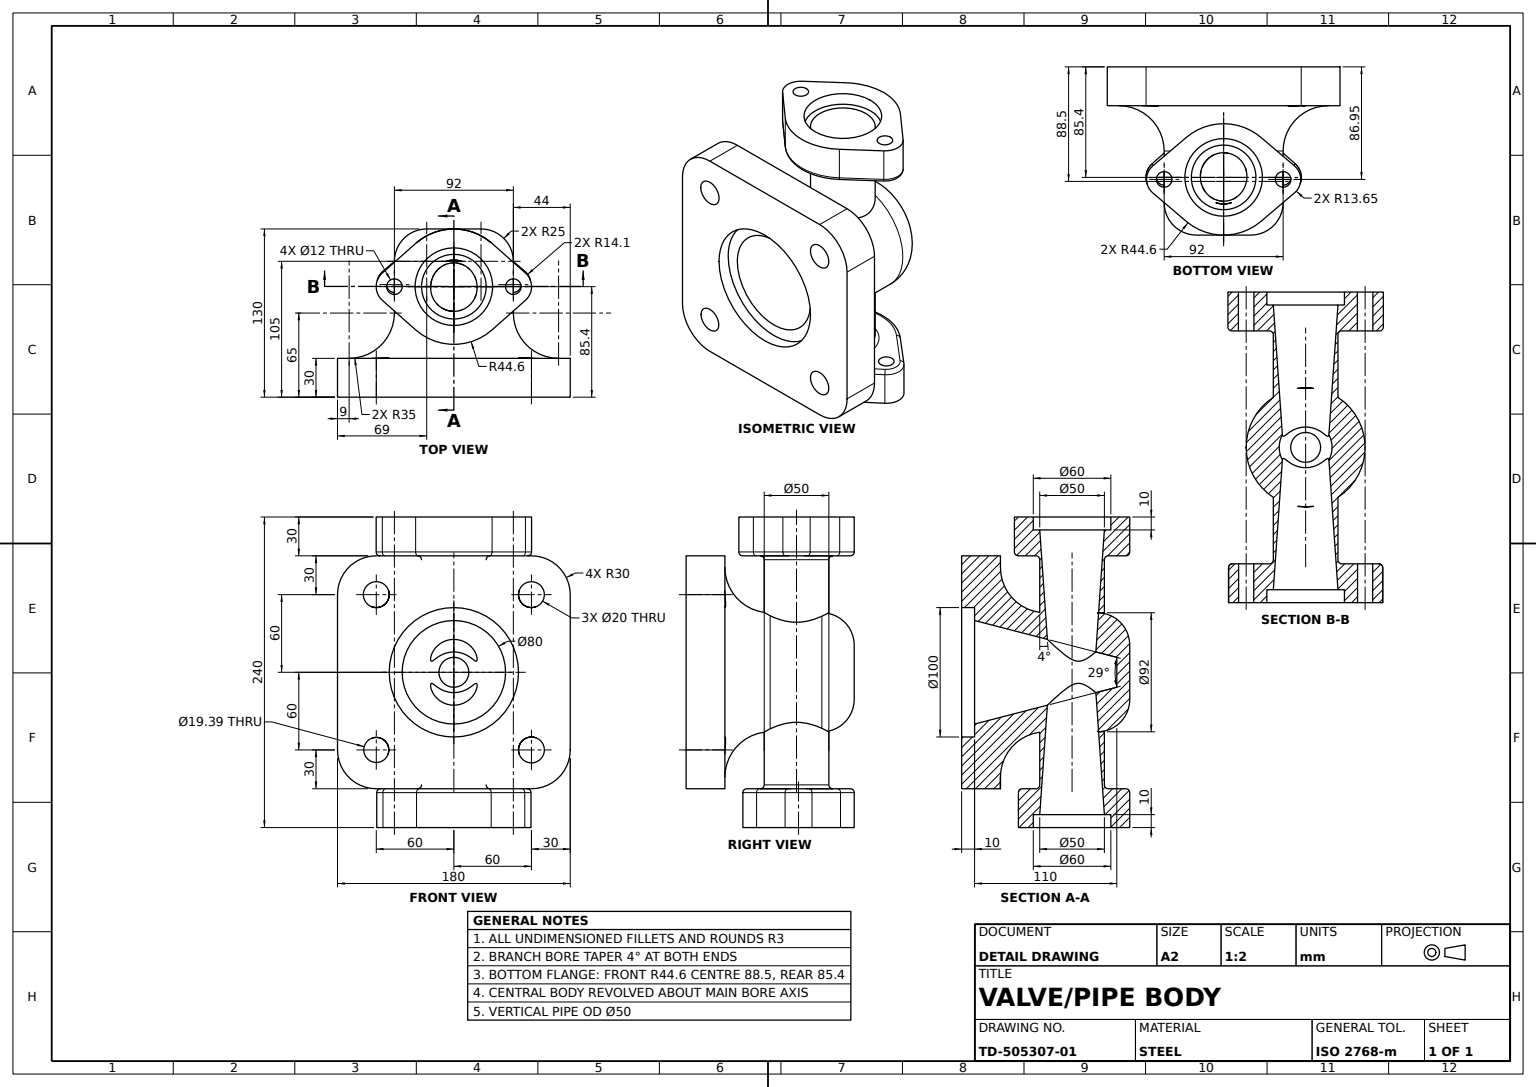
from build123d import *

# Parameters (mm, degrees)
SQUARE_FLANGE_SKETCH_W          = 180
SQUARE_FLANGE_SKETCH_H          = 180
SQUARE_FLANGE_180X180_DEPTH     = 30
FLANGE_CORNER_FILLETS_R30_R     = 30
OVAL_FLANGE_A_SKETCH_R          = 6
OVAL_FLANGE_A_DEPTH             = 30
OVAL_FLANGE_B_SKETCH_R          = 6
OVAL_FLANGE_B_DEPTH             = 30
FLANGE_B_COUNTERBORE_SKETCH_R   = 30
FLANGE_B_COUNTERBORE_60_DEPTH   = 10
FLANGE_A_COUNTERBORE_SKETCH_R   = 30
FLANGE_A_COUNTERBORE_60_DEPTH   = 10
MAIN_PORT_COUNTERBORE_SKETCH_R  = 50
MAIN_PORT_COUNTERBORE_100_DEPTH = 10
MAIN_BORE_SKETCH_R              = 40
MAIN_TAPERED_BORE_80_DEPTH      = 110
MAIN_TAPERED_BORE_80_DRAFT      = -14.5
BRANCH_NECK_B_50_REACH          = 251.399
BRANCH_NECK_B_50_END_RADIUS     = 46
BRANCH_NECK_B_SKETCH_R          = 25
BRANCH_NECK_A_50_REACH          = 251.399
BRANCH_NECK_A_50_END_RADIUS     = 46
BRANCH_NECK_A_SKETCH_R          = 25
BRANCH_BORE_B_SKETCH_R          = 25
BRANCH_TAPERED_BORE_B_50_DEPTH  = 110
BRANCH_TAPERED_BORE_B_50_DRAFT  = -4
BRANCH_BORE_A_SKETCH_R          = 25
BRANCH_TAPERED_BORE_A_50_DEPTH  = 110
BRANCH_TAPERED_BORE_A_50_DRAFT  = -4
OVAL_FLANGE_FILLETS_R3_R        = 3
BRANCH_NECK_FILLETS_R3_R        = 3
RELIEF_CUT_12X12_SKETCH_R       = 6
RELIEF_CUT_12X12_DEPTH          = 15
RELIEF_CUT_20X20_SKETCH_R       = 10
RELIEF_CUT_20X20_SKETCH_R_2     = 9.692621227
RELIEF_CUT_20X20_DEPTH          = 35


with BuildPart() as part:
    # Square Flange Sketch → Square Flange 180x180 (new body)
    with BuildSketch(Plane.XY):
        Rectangle(SQUARE_FLANGE_SKETCH_W, SQUARE_FLANGE_SKETCH_H)
    extrude(amount=SQUARE_FLANGE_180X180_DEPTH)

    # Flange Corner Fillets R30
    flange_corner_fillets_r30_edges = [part.edges().sort_by_distance(p)[0] for p in [
        (90, -90, 15),
        (-90, -90, 15),
        (-90, 90, 15),
        (90, 90, 15),
    ]]
    fillet(flange_corner_fillets_r30_edges, radius=FLANGE_CORNER_FILLETS_R30_R)

    # Tee Body Profile Sketch → Tee Body Revolve (revolve)
    with BuildSketch(Plane(origin=(0, 0, 0), x_dir=(1, 0, 0), z_dir=(0, 1, 0)), mode=Mode.PRIVATE) as tee_body_revolve_sk:
        with BuildLine():
            Line((0, 100), (21, 100))
            ThreePointArc((21, 100), (38.67766953, 92.67766953), (46, 75))
            Line((46, 75), (46, 35))
            ThreePointArc((46, 35), (56.251262658, 10.251262658), (81, 0))
            Line((81, 0), (0, 0))
            Line((0, 0), (0, 100))
        make_face()
    revolve(tee_body_revolve_sk.sketch.rotate(Axis((0, 0, -100), (0, 0, 1)), 180), axis=Axis((0, 0, -100), (0, 0, 1)))

    # Main Port Counterbore Sketch → Main Port Counterbore Ø100 (cut)
    with BuildSketch(Plane.XY.offset(30)):
        Circle(MAIN_PORT_COUNTERBORE_SKETCH_R)
    extrude(amount=-MAIN_PORT_COUNTERBORE_100_DEPTH, mode=Mode.SUBTRACT)


with BuildPart() as body_2:
    # Oval Flange A Sketch → Oval Flange A (new body)
    with BuildSketch(Plane.XZ.offset(90)):
        with BuildLine():
            Line((-28.86179798, -24.498439995), (-54.833424184, -46.543647524))
            ThreePointArc((-54.833424184, -46.543647524), (-59.650248639, -56.950371557), (-54.833424184, -67.35709559))
            Line((-54.833424184, -67.35709559), (-28.86179798, -89.402303119))
            ThreePointArc((-28.86179798, -89.402303119), (0, -100), (28.86179798, -89.402303119))
            Line((28.86179798, -89.402303119), (54.833424184, -67.35709559))
            ThreePointArc((54.833424184, -67.35709559), (59.650248639, -56.950371557), (54.833424184, -46.543647524))
            Line((54.833424184, -46.543647524), (28.86179798, -24.498439995))
            ThreePointArc((28.86179798, -24.498439995), (0, -13.900743113), (-28.86179798, -24.498439995))
        make_face()
        with Locations(Location((-46, -56.950371557, 0), (0, 0, 270))):
            Circle(OVAL_FLANGE_A_SKETCH_R, mode=Mode.SUBTRACT)
        with Locations(Location((46, -56.950371557, 0), (0, 0, 270))):
            Circle(OVAL_FLANGE_A_SKETCH_R, mode=Mode.SUBTRACT)
    extrude(amount=OVAL_FLANGE_A_DEPTH)

    # Flange A Counterbore Sketch → Flange A Counterbore Ø60 (cut)
    with BuildSketch(Plane.XZ.offset(120)):
        with Locations(Location((0, -55.4, 0), (0, 0, 270))):
            Circle(FLANGE_A_COUNTERBORE_SKETCH_R)
    extrude(amount=-FLANGE_A_COUNTERBORE_60_DEPTH, mode=Mode.SUBTRACT)


with BuildPart() as body_3:
    # Oval Flange B Sketch → Oval Flange B (new body)
    with BuildSketch(Plane(origin=(0, 90, 0), x_dir=(1, 0, 0), z_dir=(0, 1, 0))):
        with BuildLine():
            Line((29.57173913, 88.786707606), (55.348913043, 65.954990521))
            ThreePointArc((55.348913043, 65.954990521), (60.1, 55.4), (55.348913043, 44.845009479))
            Line((55.348913043, 44.845009479), (29.57173913, 22.013292394))
            ThreePointArc((29.57173913, 22.013292394), (0, 10.8), (-29.57173913, 22.013292394))
            Line((-29.57173913, 22.013292394), (-55.348913043, 44.845009479))
            ThreePointArc((-55.348913043, 44.845009479), (-60.1, 55.4), (-55.348913043, 65.954990521))
            Line((-55.348913043, 65.954990521), (-29.57173913, 88.786707606))
            ThreePointArc((-29.57173913, 88.786707606), (0, 100), (29.57173913, 88.786707606))
        make_face()
        with Locations(Location((-46, 55.4, 0), (0, 0, 270))):
            Circle(OVAL_FLANGE_B_SKETCH_R, mode=Mode.SUBTRACT)
        with Locations(Location((46, 55.4, 0), (0, 0, 270))):
            Circle(OVAL_FLANGE_B_SKETCH_R, mode=Mode.SUBTRACT)
    extrude(amount=OVAL_FLANGE_B_DEPTH)

    # Flange B Counterbore Sketch → Flange B Counterbore Ø60 (cut)
    with BuildSketch(Plane(origin=(0, 120, 0), x_dir=(1, 0, 0), z_dir=(0, 1, 0))):
        with Locations(Location((0, 55.4, 0), (0, 0, 270))):
            Circle(FLANGE_B_COUNTERBORE_SKETCH_R)
    extrude(amount=-FLANGE_B_COUNTERBORE_60_DEPTH, mode=Mode.SUBTRACT)


with BuildPart() as main_tapered_bore_80_tool:
    # Main Bore Sketch → Main Tapered Bore Ø80 (with draft: the straight prism first)
    with BuildSketch(Plane.XY.offset(20)):
        Circle(MAIN_BORE_SKETCH_R)
    extrude(amount=-MAIN_TAPERED_BORE_80_DEPTH)
    # Main Tapered Bore Ø80: the draft: its side faces are tilted about the plane it starts from
    main_tapered_bore_80_sides = [main_tapered_bore_80_tool.faces().sort_by_distance(p)[0] for p in [
        (-40, 0, -35),
    ]]
    draft(main_tapered_bore_80_sides, Plane.XY.offset(20), MAIN_TAPERED_BORE_80_DRAFT)


with BuildPart() as part_1:
    add(part.part)

    # Main Tapered Bore Ø80: cut by main_tapered_bore_80_tool
    add(main_tapered_bore_80_tool.part, mode=Mode.SUBTRACT)


    add(body_3.part)  # Branch Neck B Ø50 merges body 3
    # Branch Neck B Ø50: up to this cylinder (the profile starts outside it)
    branch_neck_b_50_end = Plane(origin=(0, 0, -55.4), z_dir=(0, 0, -1)) * Cylinder(BRANCH_NECK_B_50_END_RADIUS, 595.798, mode=Mode.PRIVATE)
    # Branch Neck B Sketch → Branch Neck B Ø50 (add, up to the surface)
    with BuildSketch(Plane.XZ.offset(-90), mode=Mode.PRIVATE) as branch_neck_b_50_sk1:
        with Locations(Location((0, -55.4, 0), (0, 0, 125.313640034))):
            Circle(BRANCH_NECK_B_SKETCH_R)
    branch_neck_b_50_tool1 = extrude(branch_neck_b_50_sk1.sketch, amount=BRANCH_NECK_B_50_REACH, mode=Mode.PRIVATE) - branch_neck_b_50_end
    add(branch_neck_b_50_tool1.solids().sort_by_distance((0, 90, -55.4))[0])


    add(body_2.part)  # Branch Neck A Ø50 merges body 2
    # Branch Neck A Ø50: up to this cylinder (the profile starts outside it)
    branch_neck_a_50_end = Plane(origin=(0, 0, -55.4), z_dir=(0, 0, -1)) * Cylinder(BRANCH_NECK_A_50_END_RADIUS, 595.798, mode=Mode.PRIVATE)
    # Branch Neck A Sketch → Branch Neck A Ø50 (add, up to the surface)
    with BuildSketch(Plane(origin=(0, -90, 0), x_dir=(1, 0, 0), z_dir=(0, 1, 0)), mode=Mode.PRIVATE) as branch_neck_a_50_sk1:
        with Locations(Location((0, 55.4, 0), (0, 0, 51.628286382))):
            Circle(BRANCH_NECK_A_SKETCH_R)
    branch_neck_a_50_tool1 = extrude(branch_neck_a_50_sk1.sketch, amount=BRANCH_NECK_A_50_REACH, mode=Mode.PRIVATE) - branch_neck_a_50_end
    add(branch_neck_a_50_tool1.solids().sort_by_distance((0, -90, -55.4))[0])


with BuildPart() as branch_tapered_bore_b_50_tool:
    # Branch Bore B Sketch → Branch Tapered Bore B Ø50 (with draft: the straight prism first)
    with BuildSketch(Plane(origin=(0, 110, 0), x_dir=(1, 0, 0), z_dir=(0, 1, 0))):
        with Locations(Location((0, 55.4, 0), (0, 0, 51.628286382))):
            Circle(BRANCH_BORE_B_SKETCH_R)
    extrude(amount=-BRANCH_TAPERED_BORE_B_50_DEPTH)
    # Branch Tapered Bore B Ø50: the draft: its side faces are tilted about the plane it starts from
    branch_tapered_bore_b_50_sides = [branch_tapered_bore_b_50_tool.faces().sort_by_distance(p)[0] for p in [
        (-15.519020065, 55, -35.799999586),
    ]]
    draft(branch_tapered_bore_b_50_sides, Plane(origin=(0, 110, 0), x_dir=(1, 0, 0), z_dir=(0, 1, 0)), BRANCH_TAPERED_BORE_B_50_DRAFT)


with BuildPart() as part_2:
    add(part_1.part)

    # Branch Tapered Bore B Ø50: cut by branch_tapered_bore_b_50_tool
    add(branch_tapered_bore_b_50_tool.part, mode=Mode.SUBTRACT)


with BuildPart() as branch_tapered_bore_a_50_tool:
    # Branch Bore A Sketch → Branch Tapered Bore A Ø50 (with draft: the straight prism first)
    with BuildSketch(Plane.XZ.offset(110)):
        with Locations(Location((0, -55.4, 0), (0, 0, 308.371713618))):
            Circle(BRANCH_BORE_A_SKETCH_R)
    extrude(amount=-BRANCH_TAPERED_BORE_A_50_DEPTH)
    # Branch Tapered Bore A Ø50: the draft: its side faces are tilted about the plane it starts from
    branch_tapered_bore_a_50_sides = [branch_tapered_bore_a_50_tool.faces().sort_by_distance(p)[0] for p in [
        (-15.519020065, -55, -35.799999586),
    ]]
    draft(branch_tapered_bore_a_50_sides, Plane.XZ.offset(110), BRANCH_TAPERED_BORE_A_50_DRAFT)


with BuildPart() as part_3:
    add(part_2.part)

    # Branch Tapered Bore A Ø50: cut by branch_tapered_bore_a_50_tool
    add(branch_tapered_bore_a_50_tool.part, mode=Mode.SUBTRACT)

    # Oval Flange Fillets R3
    oval_flange_fillets_r3_edges = [part_3.edges().sort_by_distance(p)[0] for p in [
        (41.847611082, -90, -35.521043759),
        (59.650248639, -90, -56.950371557),
        (41.847611082, -90, -78.379699354),
        (0, -90, -100),
        (0, 90, -10.8),
        (42.460326087, 90, -33.429150936),
        (60.1, 90, -55.4),
        (42.460326087, 90, -77.370849064),
        (0, 90, -100),
        (-42.460326087, 90, -77.370849064),
        (-60.1, 90, -55.4),
        (-42.460326087, 90, -33.429150936),
        (-41.847611082, -90, -78.379699354),
        (-59.650248639, -90, -56.950371557),
        (-41.847611082, -90, -35.521043759),
        (0, -90, -13.900743113),
    ]]
    fillet(oval_flange_fillets_r3_edges, radius=OVAL_FLANGE_FILLETS_R3_R)

    # Branch Neck Fillets R3
    branch_neck_fillets_r3_edges = [part_3.edges().sort_by_distance(p)[0] for p in [
        (-15.519020065, -90, -35.799999586),
        (14.451297515, 90, -75.800000004),
    ]]
    fillet(branch_neck_fillets_r3_edges, radius=BRANCH_NECK_FILLETS_R3_R)

    # Relief Cut 12x12 Sketch → Relief Cut 12x12 (cut)
    with BuildSketch(Plane.XY.offset(30)):
        with Locations((-60, 60)):
            Circle(RELIEF_CUT_12X12_SKETCH_R)
        with Locations((60, 60)):
            Circle(RELIEF_CUT_12X12_SKETCH_R)
        with Locations(Location((60, -60, 0), (0, 0, 180))):
            Circle(RELIEF_CUT_12X12_SKETCH_R)
        with Locations(Location((-60, -60, 0), (0, 0, 180))):
            Circle(RELIEF_CUT_12X12_SKETCH_R)
    extrude(amount=-RELIEF_CUT_12X12_DEPTH, mode=Mode.SUBTRACT)

    # Relief Cut 20x20 Sketch → Relief Cut 20x20 (cut)
    with BuildSketch(Plane.XY.offset(30)):
        with Locations((-60, 60)):
            Circle(RELIEF_CUT_20X20_SKETCH_R)
        with Locations((60, 60)):
            Circle(RELIEF_CUT_20X20_SKETCH_R)
        with Locations((-60, -60)):
            Circle(RELIEF_CUT_20X20_SKETCH_R_2)
        with Locations((60, -60)):
            Circle(RELIEF_CUT_20X20_SKETCH_R)
    extrude(amount=-RELIEF_CUT_20X20_DEPTH, mode=Mode.SUBTRACT)


solid = part_3.part
